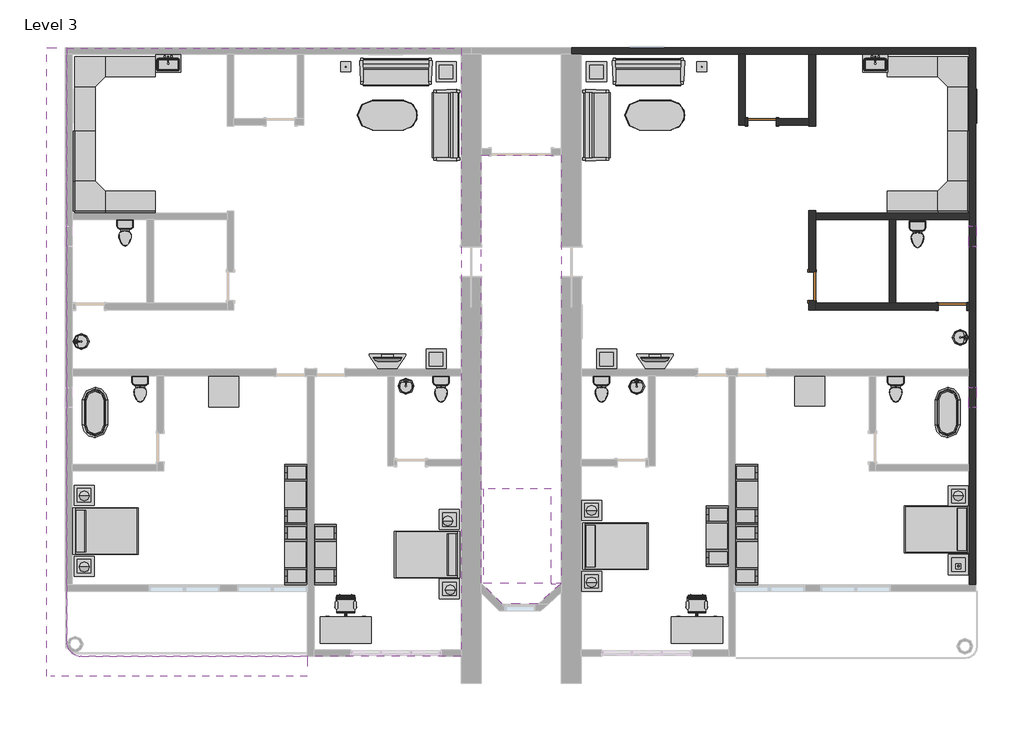
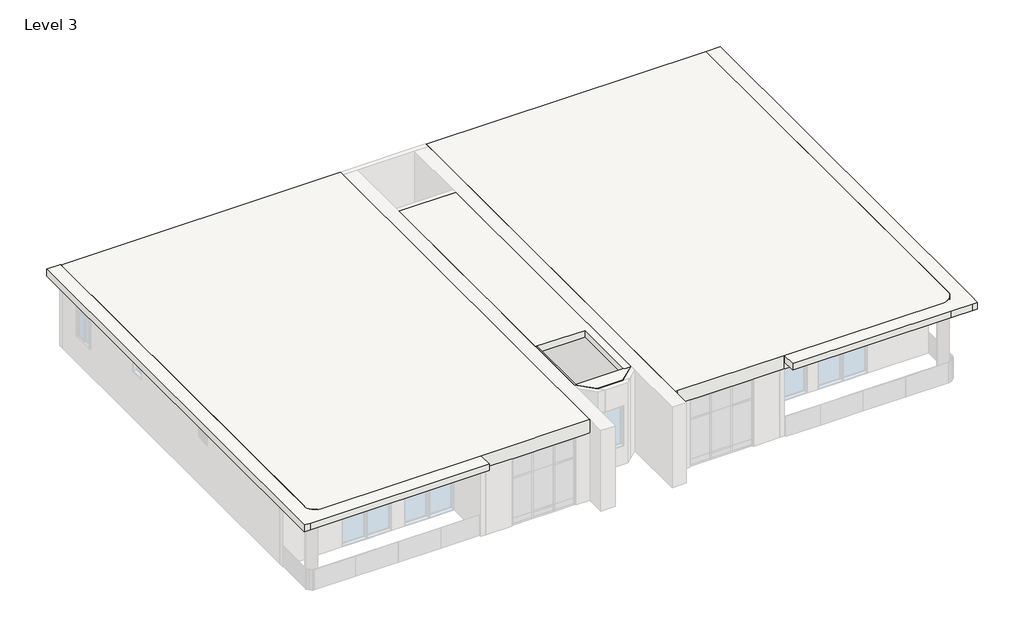
# One storey, part 3 of 3: 42 furniture elements, 14 flow terminals, 10 light fixtures, 9 walls, 4 slabs, 3 doors, 3 windows.
# Revit data of these elements (continued)
# Elements 34, 35, 36, 37 (IfcFurniture, "Sofa-Pensi : 84\"")
#   Phase Created = New Construction
#   Materials on its faces: "Cherry", "Linen, Beige", "Steel, Chrome Plated"
# Elements 38, 39 (IfcFurniture, "TV - Flat Screen : 32\"")
#   Stand = yes
#   Phase Created = New Construction
#   Materials on its faces: "TV - Black", "TV - Glass", "TV - Screen"
# Elements 40, 41 (IfcFurniture, "TV Stand : TV Stand")
#   Phase Created = New Construction
#   Materials on its faces: "Melamine - Gray", "Glass - Shelves"
# Elements 42, 43, 44, 45, 46, 47, 48, 49, 50, 51, 52, 53 (IfcFurniture, "Table-Coffee : 24\" x 24\" x 24\"")
#   Phase Created = New Construction
#   Materials on its faces: "Glass - Clear, Grey"
# Elements 54, 55 (IfcFurniture, "Table-Dining Oval : 36\" x 72\"")
#   Phase Created = New Construction
#   Materials on its faces: "Steel, Chrome Plated", "Glass - Clear, Grey"
# Elements 56, 57 (IfcFurniture, "Table-Rectangular : 36\" x 36\"")
#   Phase Created = New Construction
#   Materials on its faces: "Birch"
# Elements 58, 59 (IfcFurniture, "Work Station Cubicle : 96\" x 96\"")
#   Phase Created = New Construction
#   Materials on its faces: "Textile - Light Gray", "Laminate, Ivory, Matte"
# Element 60 (IfcLightFixture, "100W - 120V")
#   Mark = "44"
#   Phase Created = New Construction
#   Materials on its faces: "Steel, Chrome Plated", "Glass, Frosted"
# Element 61 (IfcLightFixture, "100W - 120V")
#   Mark = "45"
#   Phase Created = New Construction
#   Materials on its faces: "Steel, Chrome Plated", "Glass, Frosted"
# Element 62 (IfcLightFixture, "Table Lamp - Hemispheric : 60W - 120V")
#   Mark = "46"
#   Phase Created = New Construction
#   Materials on its faces: "Steel, Chrome Plated", "Glass, Frosted", "Birch"
# Element 63 (IfcLightFixture, "Table Lamp - Hemispheric : 60W - 120V")
#   Mark = "47"
#   Phase Created = New Construction
#   Materials on its faces: "Steel, Chrome Plated", "Glass, Frosted", "Birch"
# Element 64 (IfcLightFixture, "Table Lamp - Hemispheric : 60W - 120V")
#   Mark = "48"
#   Phase Created = New Construction
#   Materials on its faces: "Steel, Chrome Plated", "Glass, Frosted", "Birch"
# Element 65 (IfcLightFixture, "Table Lamp - Hemispheric : 60W - 120V")
#   Mark = "49"
#   Phase Created = New Construction
#   Materials on its faces: "Steel, Chrome Plated", "Glass, Frosted", "Birch"
# Element 66 (IfcLightFixture, "Table Lamp - Hemispheric : 60W - 120V")
#   Mark = "50"
#   Phase Created = New Construction
#   Materials on its faces: "Steel, Chrome Plated", "Glass, Frosted", "Birch"
# Element 67 (IfcLightFixture, "Table Lamp - Hemispheric : 60W - 120V")
#   Mark = "51"
#   Phase Created = New Construction
#   Materials on its faces: "Steel, Chrome Plated", "Glass, Frosted", "Birch"
# Element 68 (IfcLightFixture, "Table Lamp - Hemispheric : 60W - 120V")
#   Mark = "52"
#   Phase Created = New Construction
#   Materials on its faces: "Steel, Chrome Plated", "Glass, Frosted", "Birch"
# Element 69 (IfcLightFixture, "Table Lamp - Hemispheric : 60W - 120V")
#   Mark = "53"
#   Phase Created = New Construction
#   Materials on its faces: "Steel, Chrome Plated", "Glass, Frosted", "Birch"
# Element 70 (IfcSlab, "Generic - 12\" cream")
#   Height Offset From Level = 12' - 0"
#   Phase Created = New Construction
#   Materials on its faces: "Parking Stripe"
# Element 71 (IfcSlab, "Generic - 12\" white")
#   built-in parameter 1001955 = 3.14159 (stored number, unit not read)
#   Height Offset From Level = 12' - 0"
#   Phase Created = New Construction
#   Materials on its faces: "Door - Frame"
# Elements 72, 73 (IfcSlab, "Generic - 12\" white")
#   Height Offset From Level = 12' - 0"
#   Phase Created = New Construction
#   Materials on its faces: "Door - Frame"
# Elements 74, 75, 76, 77, 78, 79, 80, 81 (IfcWall, "Generic - 8\" cream")
#   Top Offset = 0' - 0"
#   Base Offset = 0' - 0"
#   Unconnected Height = 10' - 0"
#   wall height = 10' - 0"
#   Phase Created = New Construction
#   Base Constraint = Level 3
#   Materials on its faces: "Parking Stripe"
# Element 82 (IfcWall, "Generic - 8\" white")
#   Top Offset = 0' - 0"
#   Base Offset = 0' - 0"
#   Unconnected Height = 10' - 0"
#   wall height = 10' - 0"
#   Phase Created = New Construction
#   Base Constraint = Level 3
#   Materials on its faces: "Door - Frame", "Parking Stripe"
# Element 83 (IfcWindow, "Louvers with Trim : 24\" x 24\"")
#   Mark = "91"
#   Phase Created = New Construction
#   Materials on its faces: "Glass", "Iron, Ductile"
# Element 84 (IfcWindow, "Louvers with Trim : 24\" x 24\"")
#   Mark = "92"
#   Phase Created = New Construction
#   Materials on its faces: "Glass", "Iron, Ductile"
# Element 85 (IfcWindow, "Slider with Trim : 36\" x 48\"")
#   Mark = "88"
#   Phase Created = New Construction
#   Materials on its faces: "Iron, Ductile", "Glass"
# Materials
#   "Wood - Birch - Solid Stained Light Low Gloss": class "Wood", colour RGB 210 159 95, transparency 0, Cost = 0
#   "Paint - Sienna": colour RGB 118 70 51, transparency 0, Cost = 0
#   "Steel, Polished": class "Metal", colour RGB 57 57 57, transparency 0, Description = "Polished steel", Cost = 0
#   "Porcelain, Linen": class "Ceramic", colour RGB 249 239 230, transparency 0, Description = "Porcelain, linen", Cost = 0
#   "Laminate, Linen, Matte": class "Plastic", colour RGB 249 239 230, transparency 0, Description = "Plastic Laminate - Linen, Matte", Cost = 0
#   "Porcelain, Ivory": class "Ceramic", colour RGB 247 247 239, transparency 0, Description = "Porcelain, ivory", Cost = 0
#   "Laminate, Ivory, Matte": class "Plastic", colour RGB 247 247 239, transparency 0, Description = "Plastic Laminate - Ivory, Matte", Cost = 0
#   "Birch": class "Wood", colour RGB 224 178 126, transparency 0, Description = "Betula Alleghaniensis", Cost = 0
#   "Linen, White": class "Textile", colour RGB 247 247 239, transparency 0, Description = "Linen, white", Cost = 0
#   "Plastic, Opaque Black": class "Plastic", colour RGB 0 0 0, transparency 0.7, Description = "Plastic, generic, opaque black", Cost = 0
#   "Textile - Slate Blue": class "Fabric", colour RGB 98 102 118, transparency 0
#   "Steel, Chrome Plated": class "Metal", colour RGB 17 17 17, transparency 0, Description = "Chromiuim plated steel", Cost = 0
#   "Cherry": class "Wood", colour RGB 226 177 128, transparency 0, Description = "Prunus Serotina", Cost = 0
#   "Linen, Beige": class "Textile", colour RGB 249 239 230, transparency 0, Description = "Linen, beige", Cost = 0
#   "Melamine - Gray": class "Wood", colour RGB 49 49 49, transparency 0
#   "Glass - Clear, Grey": class "Glass", colour RGB 252 255 255, transparency 0.64
#   "Textile - Light Gray": class "Fabric", colour RGB 204 204 204, transparency 0
#   "Glass, Frosted": class "Glass", colour RGB 250 244 225, transparency 0.55, Description = "physical material", Cost = 0
#   "Parking Stripe": class "Paint", colour RGB 250 250 91, transparency 0, Cost = 0
#   "Door - Frame": colour RGB 118 70 51, transparency 0, Cost = 0
#   "Iron, Ductile": class "Metal", colour RGB 0 0 0, transparency 0, Description = "Ductile cast iron", Cost = 0
#   "Glass": class "Glass", colour RGB 0 128 192, transparency 0.75, Description = "Soda Lime Glass", Cost = 0
#   "TV - Black": colour RGB 49 49 49, transparency 0
#   "TV - Glass": colour RGB 157 157 157, transparency 0.9
#   "TV - Screen": colour RGB 0 0 0, transparency 0
#   "Glass - Shelves": class "Glass", colour RGB 167 167 167, transparency 0.9
